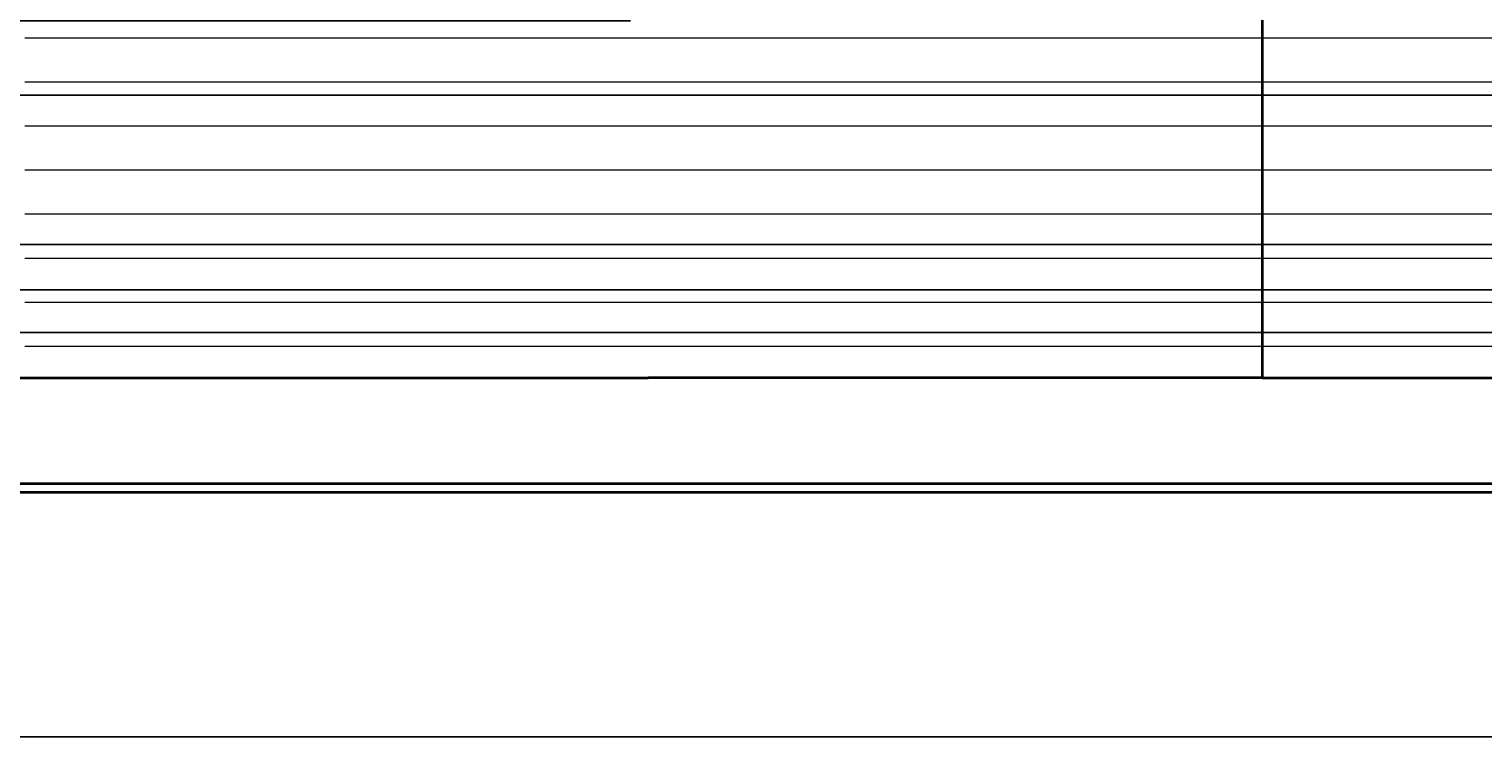
# Model space of a CAD drawing. Units: inches. Extents: x -30 to 1188, y 40 to 520.
# Tile 5 of 7: x 656 to 986, y 40 to 202. Entities that reach past the tile are written whole.
import ezdxf

# ---------------------------------------------------------------- set-up
doc = ezdxf.new("R2010")
doc.units = ezdxf.units.IN
doc.header["$MEASUREMENT"] = 0
for name, color, linetype, lineweight in [('A-ANNO-DIMS', 2, 'Continuous', 18), ('A-ELEV', 7, 'Continuous', 35), ('A-ELEV-PATT', 8, 'Continuous', 13)]:
    doc.layers.add(name, color=color, linetype=linetype, lineweight=lineweight)
doc.styles.get("Standard").update_dxf_attribs({"font": 'arial.ttf'})
doc.dimstyles.get("Standard").update_dxf_attribs({"dimtxt": 2.0625, "dimasz": 0.18, "dimexe": 0.18, "dimexo": 0.0625, "dimgap": 0.09, "dimtad": 0, "dimtih": 1, "dimtoh": 1, "dimdec": 4, "dimzin": 0, "dimdsep": 46, "dimlunit": 4, "dimtxsty": 'Standard', "dimcen": 0.09, "dimadec": 0, "dimazin": 0, "dimtfac": 1, "dimtdec": 4, "dimtofl": 0, "dimtmove": 0, "dimatfit": 3, "dimfxl": 1, "dimtolj": 1, "dimtzin": 0, "dimarcsym": 0})

# ---------------------------------------------------------------- blocks, each defined once
blk = doc.blocks.new('*D4')
at = {"layer": 'A-ANNO-DIMS', "color": 0, "lineweight": -2, "transparency": 16777216}
for p, q in [((73.66, 122.81), (73.66, 41.19)), ((1107.88, 118.31), (1107.88, 41.19)), ((73.84, 41.37), (586.5, 41.37)), ((1107.7, 41.37), (595.03, 41.37))]:
    blk.add_line(p, q, dxfattribs=at)
at = {"layer": 'A-ANNO-DIMS', "color": 0, "transparency": 16777216}
for points in [[(73.84, 41.4), (73.84, 41.34), (73.66, 41.37)], [(1107.7, 41.4), (1107.7, 41.34), (1107.88, 41.37)]]:
    blk.add_solid(points, dxfattribs=at)
at = {"layer": 'Defpoints', "color": 0, "transparency": 16777216}
for p in [(73.66, 122.87), (1107.88, 118.38), (1107.88, 41.37)]:
    blk.add_point(p, dxfattribs=at)
at = {"layer": 'A-ANNO-DIMS', "color": 0, "transparency": 16777216, "insert": (590.77, 41.37), "char_height": 2.062, "attachment_point": 5}
blk.add_mtext('\\A1;1034.2', dxfattribs=at)
blk = doc.blocks.new('*D31')
at = {"layer": 'A-ANNO-DIMS', "color": 0, "lineweight": -2, "transparency": 16777216}
for p, q in [((792.57, 203.84), (-25.83, 203.84)), ((-25.65, 203.66), (-25.65, 164.5)), ((-25.65, 123.05), (-25.65, 162.21)), ((935.84, 122.87), (-25.83, 122.87))]:
    blk.add_line(p, q, dxfattribs=at)
at = {"layer": 'A-ANNO-DIMS', "color": 0, "transparency": 16777216}
for points in [[(-25.68, 203.66), (-25.62, 203.66), (-25.65, 203.84)], [(-25.68, 123.05), (-25.62, 123.05), (-25.65, 122.87)]]:
    blk.add_solid(points, dxfattribs=at)
at = {"layer": 'Defpoints', "color": 0, "transparency": 16777216}
for p in [(792.63, 203.84), (-25.65, 122.87), (935.9, 122.87)]:
    blk.add_point(p, dxfattribs=at)
at = {"layer": 'A-ANNO-DIMS', "color": 0, "transparency": 16777216, "insert": (-25.65, 163.36), "char_height": 2.062, "attachment_point": 5}
blk.add_mtext('\\A1;80.97', dxfattribs=at)
blk = doc.blocks.new('*D35')
at = {"layer": 'A-ANNO-DIMS', "color": 0, "lineweight": -2, "transparency": 16777216}
for p, q in [((99.49, 122.87), (1183.93, 122.87)), ((1183.75, 122.69), (1183.75, 112)), ((1183.75, 99.05), (1183.75, 109.75)), ((99.49, 98.87), (1183.93, 98.87))]:
    blk.add_line(p, q, dxfattribs=at)
at = {"layer": 'A-ANNO-DIMS', "color": 0, "transparency": 16777216}
for points in [[(1183.72, 122.69), (1183.78, 122.69), (1183.75, 122.87)], [(1183.72, 99.05), (1183.78, 99.05), (1183.75, 98.87)]]:
    blk.add_solid(points, dxfattribs=at)
at = {"layer": 'Defpoints', "color": 0, "transparency": 16777216}
for p in [(99.43, 122.87), (1183.75, 122.87), (99.43, 98.87)]:
    blk.add_point(p, dxfattribs=at)
at = {"layer": 'A-ANNO-DIMS', "color": 0, "transparency": 16777216, "insert": (1183.75, 110.87), "char_height": 2.062, "attachment_point": 5}
blk.add_mtext('\\A1;24', dxfattribs=at)
blk = doc.blocks.new('*D36')
at = {"layer": 'A-ANNO-DIMS', "color": 0, "lineweight": -2, "transparency": 16777216}
for p, q in [((99.49, 133.14), (1183.93, 133.14)), ((1183.75, 132.96), (1183.75, 129.15)), ((1183.75, 123.05), (1183.75, 126.86)), ((99.49, 122.87), (1183.93, 122.87))]:
    blk.add_line(p, q, dxfattribs=at)
at = {"layer": 'A-ANNO-DIMS', "color": 0, "transparency": 16777216}
for points in [[(1183.72, 132.96), (1183.78, 132.96), (1183.75, 133.14)], [(1183.72, 123.05), (1183.78, 123.05), (1183.75, 122.87)]]:
    blk.add_solid(points, dxfattribs=at)
at = {"layer": 'Defpoints', "color": 0, "transparency": 16777216}
for p in [(99.43, 133.14), (1183.75, 133.14), (99.43, 122.87)]:
    blk.add_point(p, dxfattribs=at)
at = {"layer": 'A-ANNO-DIMS', "color": 0, "transparency": 16777216, "insert": (1183.75, 128.01), "char_height": 2.062, "attachment_point": 5}
blk.add_mtext('\\A1;10.268', dxfattribs=at)
blk = doc.blocks.new('*D37')
at = {"layer": 'A-ANNO-DIMS', "color": 0, "lineweight": -2, "transparency": 16777216}
for p, q in [((99.49, 186.93), (1183.93, 186.93)), ((1183.75, 186.75), (1183.75, 161.18)), ((1183.75, 133.32), (1183.75, 158.89)), ((99.49, 133.14), (1183.93, 133.14))]:
    blk.add_line(p, q, dxfattribs=at)
at = {"layer": 'A-ANNO-DIMS', "color": 0, "transparency": 16777216}
for points in [[(1183.72, 186.75), (1183.78, 186.75), (1183.75, 186.93)], [(1183.72, 133.32), (1183.78, 133.32), (1183.75, 133.14)]]:
    blk.add_solid(points, dxfattribs=at)
at = {"layer": 'Defpoints', "color": 0, "transparency": 16777216}
for p in [(99.43, 186.93), (1183.75, 186.93), (99.43, 133.14)]:
    blk.add_point(p, dxfattribs=at)
at = {"layer": 'A-ANNO-DIMS', "color": 0, "transparency": 16777216, "insert": (1183.75, 160.03), "char_height": 2.062, "attachment_point": 5}
blk.add_mtext('\\A1;53.79', dxfattribs=at)
blk = doc.blocks.new('*D38')
at = {"layer": 'A-ANNO-DIMS', "color": 0, "lineweight": -2, "transparency": 16777216}
for p, q in [((99.49, 242.87), (1183.93, 242.87)), ((1183.75, 242.69), (1183.75, 216.04)), ((1183.75, 187.11), (1183.75, 213.76)), ((99.49, 186.93), (1183.93, 186.93))]:
    blk.add_line(p, q, dxfattribs=at)
at = {"layer": 'A-ANNO-DIMS', "color": 0, "transparency": 16777216}
for points in [[(1183.72, 242.69), (1183.78, 242.69), (1183.75, 242.87)], [(1183.72, 187.11), (1183.78, 187.11), (1183.75, 186.93)]]:
    blk.add_solid(points, dxfattribs=at)
at = {"layer": 'Defpoints', "color": 0, "transparency": 16777216}
for p in [(99.43, 242.87), (1183.75, 242.87), (99.43, 186.93)]:
    blk.add_point(p, dxfattribs=at)
at = {"layer": 'A-ANNO-DIMS', "color": 0, "transparency": 16777216, "insert": (1183.75, 214.9), "char_height": 2.062, "attachment_point": 5}
blk.add_mtext('\\A1;55.94', dxfattribs=at)
blk = doc.blocks.new('*D39')
at = {"layer": 'A-ANNO-DIMS', "color": 0, "lineweight": -2, "transparency": 16777216}
for p, q in [((358.49, 186.93), (1183.93, 186.93)), ((1183.75, 186.75), (1183.75, 161.18)), ((1183.75, 133.32), (1183.75, 158.89)), ((358.49, 133.14), (1183.93, 133.14))]:
    blk.add_line(p, q, dxfattribs=at)
at = {"layer": 'A-ANNO-DIMS', "color": 0, "transparency": 16777216}
for points in [[(1183.72, 186.75), (1183.78, 186.75), (1183.75, 186.93)], [(1183.72, 133.32), (1183.78, 133.32), (1183.75, 133.14)]]:
    blk.add_solid(points, dxfattribs=at)
at = {"layer": 'Defpoints', "color": 0, "transparency": 16777216}
for p in [(358.42, 186.93), (1183.75, 186.93), (358.42, 133.14)]:
    blk.add_point(p, dxfattribs=at)
at = {"layer": 'A-ANNO-DIMS', "color": 0, "transparency": 16777216, "insert": (1183.75, 160.03), "char_height": 2.062, "attachment_point": 5}
blk.add_mtext('\\A1;53.79', dxfattribs=at)
blk = doc.blocks.new('*D40')
at = {"layer": 'A-ANNO-DIMS', "color": 0, "lineweight": -2, "transparency": 16777216}
for p, q in [((358.49, 242.87), (1183.93, 242.87)), ((1183.75, 242.69), (1183.75, 216.04)), ((1183.75, 187.11), (1183.75, 213.76)), ((358.49, 186.93), (1183.93, 186.93))]:
    blk.add_line(p, q, dxfattribs=at)
at = {"layer": 'A-ANNO-DIMS', "color": 0, "transparency": 16777216}
for points in [[(1183.72, 242.69), (1183.78, 242.69), (1183.75, 242.87)], [(1183.72, 187.11), (1183.78, 187.11), (1183.75, 186.93)]]:
    blk.add_solid(points, dxfattribs=at)
at = {"layer": 'Defpoints', "color": 0, "transparency": 16777216}
for p in [(358.42, 242.87), (1183.75, 242.87), (358.42, 186.93)]:
    blk.add_point(p, dxfattribs=at)
at = {"layer": 'A-ANNO-DIMS', "color": 0, "transparency": 16777216, "insert": (1183.75, 214.9), "char_height": 2.062, "attachment_point": 5}
blk.add_mtext('\\A1;55.94', dxfattribs=at)
blk = doc.blocks.new('*D61')
at = {"layer": 'A-ANNO-DIMS', "color": 0, "lineweight": -2, "transparency": 16777216}
for p, q in [((653.09, 208.22), (1183.93, 208.22)), ((1183.75, 208.04), (1183.75, 176.65)), ((1183.75, 142.98), (1183.75, 174.36)), ((652.92, 142.8), (1183.93, 142.8))]:
    blk.add_line(p, q, dxfattribs=at)
at = {"layer": 'A-ANNO-DIMS', "color": 0, "transparency": 16777216}
for points in [[(1183.72, 208.04), (1183.78, 208.04), (1183.75, 208.22)], [(1183.72, 142.98), (1183.78, 142.98), (1183.75, 142.8)]]:
    blk.add_solid(points, dxfattribs=at)
at = {"layer": 'Defpoints', "color": 0, "transparency": 16777216}
for p in [(653.03, 208.22), (1183.75, 208.22), (652.86, 142.8)]:
    blk.add_point(p, dxfattribs=at)
at = {"layer": 'A-ANNO-DIMS', "color": 0, "transparency": 16777216, "insert": (1183.75, 175.51), "char_height": 2.062, "attachment_point": 5}
blk.add_mtext('\\A1;65.42', dxfattribs=at)
blk = doc.blocks.new('*D63')
at = {"layer": 'A-ANNO-DIMS', "color": 0, "lineweight": -2, "transparency": 16777216}
for p, q in [((576.85, 153.08), (1183.93, 153.08)), ((1183.75, 152.9), (1183.75, 149.08)), ((1183.75, 142.98), (1183.75, 146.8)), ((588.03, 142.8), (1183.93, 142.8))]:
    blk.add_line(p, q, dxfattribs=at)
at = {"layer": 'A-ANNO-DIMS', "color": 0, "transparency": 16777216}
for points in [[(1183.72, 152.9), (1183.78, 152.9), (1183.75, 153.08)], [(1183.72, 142.98), (1183.78, 142.98), (1183.75, 142.8)]]:
    blk.add_solid(points, dxfattribs=at)
at = {"layer": 'Defpoints', "color": 0, "transparency": 16777216}
for p in [(576.78, 153.08), (587.97, 142.8), (1183.75, 142.8)]:
    blk.add_point(p, dxfattribs=at)
at = {"layer": 'A-ANNO-DIMS', "color": 0, "transparency": 16777216, "insert": (1183.75, 147.94), "char_height": 2.062, "attachment_point": 5}
blk.add_mtext('\\A1;10.286', dxfattribs=at)
blk = doc.blocks.new('*D64')
at = {"layer": 'A-ANNO-DIMS', "color": 0, "lineweight": -2, "transparency": 16777216}
for p, q in [((576.85, 245.17), (1183.93, 245.17)), ((1183.75, 244.99), (1183.75, 200.27)), ((1183.75, 153.26), (1183.75, 197.98)), ((576.85, 153.08), (1183.93, 153.08))]:
    blk.add_line(p, q, dxfattribs=at)
at = {"layer": 'A-ANNO-DIMS', "color": 0, "transparency": 16777216}
for points in [[(1183.72, 244.99), (1183.78, 244.99), (1183.75, 245.17)], [(1183.72, 153.26), (1183.78, 153.26), (1183.75, 153.08)]]:
    blk.add_solid(points, dxfattribs=at)
at = {"layer": 'Defpoints', "color": 0, "transparency": 16777216}
for p in [(576.78, 245.17), (1183.75, 245.17), (576.78, 153.08)]:
    blk.add_point(p, dxfattribs=at)
at = {"layer": 'A-ANNO-DIMS', "color": 0, "transparency": 16777216, "insert": (1183.75, 199.12), "char_height": 2.062, "attachment_point": 5}
blk.add_mtext('\\A1;92.08', dxfattribs=at)
blk = doc.blocks.new('*D74')
at = {"layer": 'A-ANNO-DIMS', "color": 0, "lineweight": -2, "transparency": 16777216}
for p, q in [((30.14, 98.93), (30.14, 518.97)), ((30.32, 518.79), (574.32, 518.79)), ((1128.07, 518.79), (584.07, 518.79)), ((1128.25, 117.62), (1128.25, 518.97))]:
    blk.add_line(p, q, dxfattribs=at)
at = {"layer": 'A-ANNO-DIMS', "color": 0, "transparency": 16777216}
for points in [[(30.32, 518.82), (30.32, 518.76), (30.14, 518.79)], [(1128.07, 518.82), (1128.07, 518.76), (1128.25, 518.79)]]:
    blk.add_solid(points, dxfattribs=at)
at = {"layer": 'Defpoints', "color": 0, "transparency": 16777216}
for p in [(1128.25, 518.79), (1128.25, 117.56), (30.14, 98.87)]:
    blk.add_point(p, dxfattribs=at)
at = {"layer": 'A-ANNO-DIMS', "color": 0, "transparency": 16777216, "insert": (579.19, 518.79), "char_height": 2.0625, "attachment_point": 5}
blk.add_mtext('\\A1;1098.11', dxfattribs=at)

msp = doc.modelspace()

# ---------------------------------------------------------------- hatches: boundary and pattern name
at = {"layer": 'A-ELEV-PATT'}
h = msp.add_hatch(dxfattribs=at)
h.set_pattern_fill('ANSI31', color=256, scale=80, angle=135)
h.paths.add_polyline_path([(935.904, 461.2934), (655.0318, 461.2934), (655.0318, 408.0708), (655.0318, 380.8615), (798.3036, 380.8615), (798.3036, 314.3348), (655.0318, 314.3348), (655.0318, 303.0545), (655.0318, 122.8714), (744.4225, 122.8714), (796.5546, 122.8714), (935.904, 122.8714), (935.904, 203.8438), (792.6322, 203.8438), (792.6322, 270.3705), (935.904, 270.3705), (935.904, 372.8284)])
h.paths.add_polyline_path([(466.9951, 434.8714), (466.9951, 461.2934), (73.6582, 461.2934), (73.6582, 434.8714), (73.6582, 410.8714), (73.6582, 266.8714), (382.4247, 266.8714), (466.9951, 266.8714)])
h.paths.add_polyline_path([(422.6392, 390.3227), (422.6392, 317.8826), (99.4312, 317.8826), (99.4312, 390.3227)], flags=16)
h.paths.add_polyline_path([(416.8376, 385.9009), (416.8376, 322.3026), (332.2885, 322.3026), (332.2885, 385.9009)], flags=0)
h.paths.add_polyline_path([(187.4151, 386.0591), (187.4151, 322.4608), (102.866, 322.4608), (102.866, 386.0591)], flags=0)
h = msp.add_hatch(dxfattribs=at)
h.set_pattern_fill('ANSI31', color=256, scale=80, angle=135)
h.paths.add_polyline_path([(1107.8751, 235.7299), (935.904, 235.7299), (935.904, 122.8714), (995.9226, 122.8714), (1107.8751, 118.3767)])

# ---------------------------------------------------------------- linework, layer by layer
at = {"layer": 'A-ELEV'}
for p, q in [((935.904, 463.2934), (935.904, 122.8714)), ((466.9951, 122.8714), (744.4225, 122.8714)), ((744.4225, 122.8714), (796.5546, 122.8714)), ((935.904, 122.8714), (796.5546, 122.8714)), ((935.904, 122.8714), (995.9226, 122.8714)), ((435.3376, 96.8714), (799.1412, 96.8714)), ((466.9951, 98.8714), (799.4646, 98.8714)), ((799.1412, 96.8714), (1115.2418, 96.8714)), ((799.4646, 98.8714), (1115.4196, 98.8714))]:
    msp.add_line(p, q, dxfattribs=at)

# ---------------------------------------------------------------- dimensions: what is measured, and where the dimension line sits
at = {"layer": 'A-ANNO-DIMS'}
for base, p1, p2, override, picture, middle in [((1128.2474, 518.7934), (30.1395, 98.8714), (1128.2474, 117.5588), {"dimdec": 2, "dimlfac": 1, "dimrnd": 0, "dimzin": 0, "dimdsep": 46, "dimlunit": 2}, '*D74', (579.1935, 518.7934)), ((1107.8751, 41.3714), (73.6582, 122.8714), (1107.8751, 118.3767), {"dimdec": 1, "dimlfac": 1, "dimrnd": 0, "dimzin": 0, "dimdsep": 46, "dimlunit": 2}, '*D4', (590.7666, 41.3714))]:
    dim = msp.add_linear_dim(base=base, p1=p1, p2=p2, dimstyle='Standard', override=override, dxfattribs=at)
    dim.commit()
    dim.dimension.update_dxf_attribs({"geometry": picture, "text_midpoint": middle})
for base, p1, p2, override, picture, middle in [((1183.7474, 245.1654), (576.7826, 153.0843), (576.7826, 245.1654), {"dimdec": 2, "dimlfac": 1, "dimrnd": 0, "dimzin": 0, "dimdsep": 46, "dimlunit": 2}, '*D64', (1183.7474, 199.1248)), ((1183.7474, 242.8714), (99.4312, 186.9265), (99.4312, 242.8714), {"dimdec": 2, "dimlfac": 1, "dimrnd": 0, "dimzin": 0, "dimdsep": 46, "dimlunit": 2}, '*D38', (1183.7474, 214.899)), ((1183.7474, 242.8714), (358.4247, 186.9265), (358.4247, 242.8714), {"dimdec": 2, "dimlfac": 1, "dimrnd": 0, "dimzin": 0, "dimdsep": 46, "dimlunit": 2}, '*D40', (1183.7474, 214.899)), ((1183.7474, 208.218), (652.8622, 142.7981), (653.0318, 208.218), {"dimdec": 2, "dimlfac": 1, "dimrnd": 0, "dimzin": 0, "dimdsep": 46, "dimlunit": 2}, '*D61', (1183.7474, 175.508)), ((-25.6484, 122.8714), (792.6322, 203.8438), (935.904, 122.8714), {"dimdec": 2, "dimlfac": 1, "dimrnd": 0, "dimzin": 0, "dimdsep": 46, "dimlunit": 2}, '*D31', (-25.6484, 163.3576)), ((1183.7474, 186.9265), (99.4312, 133.1393), (99.4312, 186.9265), {"dimdec": 2, "dimlfac": 1, "dimrnd": 0, "dimzin": 0, "dimdsep": 46, "dimlunit": 2}, '*D37', (1183.7474, 160.0329)), ((1183.7474, 186.9265), (358.4247, 133.1393), (358.4247, 186.9265), {"dimdec": 2, "dimlfac": 1, "dimrnd": 0, "dimzin": 0, "dimdsep": 46, "dimlunit": 2}, '*D39', (1183.7474, 160.0329)), ((1183.7474, 142.7981), (576.7826, 153.0843), (587.9675, 142.7981), {"dimdec": 3, "dimlfac": 1, "dimrnd": 0, "dimzin": 0, "dimdsep": 46, "dimlunit": 2}, '*D63', (1183.7474, 147.9412)), ((1183.7474, 133.1393), (99.4312, 122.8714), (99.4312, 133.1393), {"dimdec": 3, "dimlfac": 1, "dimrnd": 0, "dimzin": 0, "dimdsep": 46, "dimlunit": 2}, '*D36', (1183.7474, 128.0054)), ((1183.7474, 122.8714), (99.4312, 98.8714), (99.4312, 122.8714), {"dimdec": 0, "dimlfac": 1, "dimrnd": 0, "dimzin": 0, "dimdsep": 46, "dimlunit": 2}, '*D35', (1183.7474, 110.8714))]:
    dim = msp.add_linear_dim(base=base, p1=p1, p2=p2, angle=90, dimstyle='Standard', override=override, dxfattribs=at)
    dim.commit()
    dim.dimension.update_dxf_attribs({"geometry": picture, "text_midpoint": middle})

doc.saveas('drawing.dxf')
